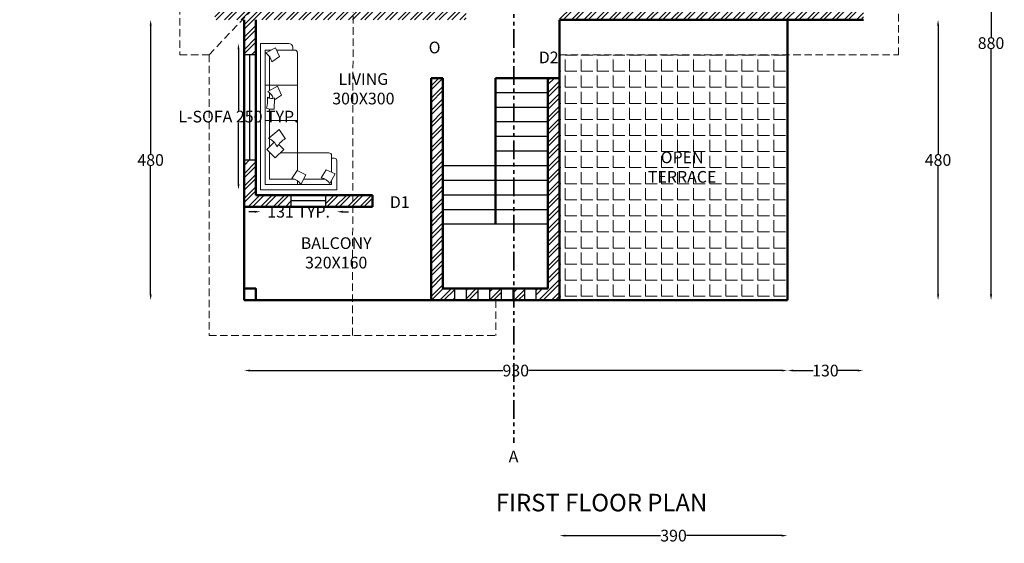
# Model space of a CAD drawing. Units: centimetres. Extents: x 10444 to 13814, y 8288 to 11191.
# Tile 8 of 9: x 12129 to 13814, y 9505 to 10401. Entities that reach past the tile are written whole.
import ezdxf

# ---------------------------------------------------------------- set-up
doc = ezdxf.new("R2010")
doc.units = ezdxf.units.CM
doc.header["$MEASUREMENT"] = 0
doc.linetypes.add('DASHED', pattern=[19.05, 12.7, -6.35])
doc.linetypes.add('PHANTOM', pattern=[63.5, 31.75, -6.35, 6.35, -6.35, 6.35, -6.35])
for name, color, linetype, lineweight in [('A-ANNO-DIMS', 2, 'Continuous', 18), ('A-ANNO-SYMB', 7, 'Continuous', 25), ('A-ANNO-SYMB-SECT', 1, 'PHANTOM', 35), ('A-ANNO-TEXT', 7, 'Continuous', 25), ('A-AREA-IDEN', 3, 'Continuous', 25), ('A-FLOR-PATT', 252, 'Continuous', 13), ('A-FLOR-STRS', 3, 'Continuous', 25), ('A-FURN', 8, 'Continuous', 18), ('A-GLAZ', 4, 'Continuous', 25), ('A-ROOF-OVHD', 6, 'DASHED', 18), ('A-WALL', 7, 'Continuous', 50), ('A-WALL-PATT', 8, 'Continuous', 13)]:
    doc.layers.add(name, color=color, linetype=linetype, lineweight=lineweight)
doc.styles.get("Standard").update_dxf_attribs({"font": 'arial.ttf'})
doc.dimstyles.get("Standard").update_dxf_attribs({"dimtxt": 20, "dimasz": 10, "dimexe": 0.18, "dimexo": 0.0625, "dimgap": 0.09, "dimtad": 0, "dimtih": 1, "dimtoh": 1, "dimdec": 0, "dimzin": 0, "dimdsep": 46, "dimtxsty": 'Standard', "dimcen": 0.09, "dimse1": 1, "dimse2": 1, "dimadec": 0, "dimazin": 0, "dimtfac": 1, "dimtdec": 0, "dimtofl": 0, "dimtmove": 0, "dimatfit": 3, "dimfxl": 1, "dimtolj": 1, "dimtzin": 0, "dimarcsym": 0})

# ---------------------------------------------------------------- blocks, each defined once
blk = doc.blocks.new('s')
at = {"color": 0, "linetype": 'ByBlock'}
for p, q in [((3164.2, 840.3), (3164.2, 844.8)), ((3171, 851.6), (3219.5, 851.6)), ((3186.7, 829.1), (3193.7, 844.2)), ((3193.7, 844.2), (3210.3, 835.3)), ((3219.5, 851.6), (3219.5, 601.2)), ((3156.3, 633.9), (3156.3, 835.8)), ((3160.9, 840.3), (3164.2, 840.3)), ((3191.9, 840.3), (3164.2, 840.3)), ((3200.2, 820.2), (3186.7, 829.1)), ((3211.6, 840.3), (3200.9, 840.3)), ((3203.7, 840.3), (3203.7, 838.8)), ((3203.7, 828.9), (3203.7, 771.1)), ((3211.6, 610.2), (3211.6, 840.3)), ((3156.3, 780.2), (3211.6, 780.2)), ((3183.2, 763.2), (3190.2, 778.3)), ((3190.2, 778.3), (3206.8, 769.4)), ((3195.3, 755.2), (3183.2, 763.2)), ((3203.7, 767.1), (3203.7, 757.8)), ((3196, 739.2), (3195.2, 758.2)), ((3203.7, 739.5), (3203.7, 674.9)), ((3156.3, 720), (3211.6, 720)), ((3187.4, 704.3), (3176.9, 688.9)), ((3205.6, 688.9), (3187.4, 704.3)), ((3188.2, 678.8), (3179.6, 670.3)), ((3208.3, 670.3), (3195.9, 682.7)), ((3097.7, 631.1), (3097.7, 659.8)), ((3102.2, 664.4), (3156.3, 664.4)), ((3156.3, 633.9), (3156.3, 664.4)), ((3156.3, 664.4), (3185.5, 664.4)), ((3179.6, 670.3), (3194, 655.9)), ((3194, 655.9), (3208.3, 670.3)), ((3203.7, 665.7), (3203.7, 619.2)), ((3088.7, 601.2), (3088.7, 650.8)), ((3093.2, 655.3), (3097.7, 655.3)), ((3106.7, 635.3), (3091.6, 628.3)), ((3091.6, 628.3), (3100.5, 611.7)), ((3115.6, 621.8), (3106.7, 635.3)), ((3156.6, 634), (3141.5, 627)), ((3141.5, 627), (3150.4, 610.4)), ((3165.5, 620.5), (3156.6, 634)), ((3097.7, 610.2), (3097.7, 616.9)), ((3156.3, 610.2), (3097.7, 610.2)), ((3145.7, 619.2), (3108.5, 619.2)), ((3156.3, 610.2), (3156.3, 616.7)), ((3156.3, 610.2), (3156.3, 616.7)), ((3211.6, 610.2), (3156.3, 610.2)), ((3203.7, 619.2), (3161.1, 619.2)), ((3156.3, 601.2), (3088.7, 601.2)), ((3219.5, 601.2), (3156.3, 601.2))]:
    blk.add_line(p, q, dxfattribs=at)
for centre, radius, start, end in [((3171, 844.8), 6.77, 90, 180), ((3160.9, 835.8), 4.51, 90, 180), ((3222.3, 816.3), 22.4, 122.3301, 170.157), ((3200.1, 772.4), 15, 250.8325, 299.9235), ((3218.8, 750.5), 22.4, 122.3301, 161.5057), ((3265.7, 754.9), 58.3, 175.599, 194.0402), ((3198.7, 772.8), 33.7, 265.4155, 288.0697), ((3153.1, 650.8), 44.9, 31.9301, 58.0699), ((3212.5, 667.6), 22.4, 108.0785, 161.9215), ((3102.2, 659.8), 4.51, 90, 180), ((3093.2, 650.8), 4.51, 90, 180), ((3119.4, 599.7), 22.4, 99.843, 147.6699), ((3169.3, 598.4), 22.4, 99.843, 147.6699)]:
    blk.add_arc(centre, radius, start, end, dxfattribs=at)
blk = doc.blocks.new('*D17')
at = {"layer": 'A-ANNO-DIMS', "color": 0, "lineweight": -2, "transparency": 16777216}
for p, q in [((12353.1, 10390.6), (12353.1, 10170.9)), ((12353.1, 9930.6), (12353.1, 10150.3))]:
    blk.add_line(p, q, dxfattribs=at)
at = {"layer": 'A-ANNO-DIMS', "color": 0, "transparency": 16777216}
for points in [[(12351.5, 10390.6), (12354.8, 10390.6), (12353.1, 10400.6)], [(12351.5, 9930.6), (12354.8, 9930.6), (12353.1, 9920.6)]]:
    blk.add_solid(points, dxfattribs=at)
at = {"layer": 'Defpoints', "color": 0, "transparency": 16777216}
for p in [(12353.1, 10400.6), (12513.1, 10400.6), (12513.1, 9920.6)]:
    blk.add_point(p, dxfattribs=at)
at = {"layer": 'A-ANNO-DIMS', "color": 0, "transparency": 16777216, "insert": (12353.1, 10160.6), "char_height": 20, "attachment_point": 5}
blk.add_mtext('\\A1;480', dxfattribs=at)
blk = doc.blocks.new('*D19')
at = {"layer": 'A-ANNO-DIMS', "color": 0, "lineweight": -2, "transparency": 16777216}
for p, q in [((13700.9, 10390.6), (13700.9, 10170.9)), ((13700.9, 9930.6), (13700.9, 10150.3))]:
    blk.add_line(p, q, dxfattribs=at)
at = {"layer": 'A-ANNO-DIMS', "color": 0, "transparency": 16777216}
for points in [[(13699.3, 10390.6), (13702.6, 10390.6), (13700.9, 10400.6)], [(13699.3, 9930.6), (13702.6, 9930.6), (13700.9, 9920.6)]]:
    blk.add_solid(points, dxfattribs=at)
at = {"layer": 'Defpoints', "color": 0, "transparency": 16777216}
for p in [(13443.1, 10400.6), (13443.1, 9920.6), (13700.9, 9920.6)]:
    blk.add_point(p, dxfattribs=at)
at = {"layer": 'A-ANNO-DIMS', "color": 0, "transparency": 16777216, "insert": (13700.9, 10160.6), "char_height": 20, "attachment_point": 5}
blk.add_mtext('\\A1;480', dxfattribs=at)
blk = doc.blocks.new('*D20')
at = {"layer": 'A-ANNO-DIMS', "color": 0, "lineweight": -2, "transparency": 16777216}
for p, q in [((12523.1, 9800.4), (12956, 9800.4)), ((13433.1, 9800.4), (13000.3, 9800.4))]:
    blk.add_line(p, q, dxfattribs=at)
at = {"layer": 'A-ANNO-DIMS', "color": 0, "transparency": 16777216}
for points in [[(12523.1, 9802.1), (12523.1, 9798.8), (12513.1, 9800.4)], [(13433.1, 9802.1), (13433.1, 9798.8), (13443.1, 9800.4)]]:
    blk.add_solid(points, dxfattribs=at)
at = {"layer": 'Defpoints', "color": 0, "transparency": 16777216}
for p in [(12513.1, 9920.6), (13443.1, 9920.6), (13443.1, 9800.4)]:
    blk.add_point(p, dxfattribs=at)
at = {"layer": 'A-ANNO-DIMS', "color": 0, "transparency": 16777216, "insert": (12978.1, 9800.4), "char_height": 20, "attachment_point": 5}
blk.add_mtext('\\A1;930', dxfattribs=at)
blk = doc.blocks.new('*D21')
at = {"layer": 'A-ANNO-DIMS', "color": 0, "lineweight": -2, "transparency": 16777216}
for p, q in [((13453.1, 9800.4), (13486.9, 9800.4)), ((13563.1, 9800.4), (13529.3, 9800.4))]:
    blk.add_line(p, q, dxfattribs=at)
at = {"layer": 'A-ANNO-DIMS', "color": 0, "transparency": 16777216}
for points in [[(13453.1, 9802.1), (13453.1, 9798.8), (13443.1, 9800.4)], [(13563.1, 9802.1), (13563.1, 9798.8), (13573.1, 9800.4)]]:
    blk.add_solid(points, dxfattribs=at)
at = {"layer": 'Defpoints', "color": 0, "transparency": 16777216}
for p in [(13443.1, 10400.6), (13573.1, 10400.6), (13443.1, 9800.4)]:
    blk.add_point(p, dxfattribs=at)
at = {"layer": 'A-ANNO-DIMS', "color": 0, "transparency": 16777216, "insert": (13508.1, 9800.4), "char_height": 20, "attachment_point": 5}
blk.add_mtext('\\A1;130', dxfattribs=at)
blk = doc.blocks.new('f')
for p, q in [((11304.7, 9881.5), (11164.7, 9881.5)), ((11164.7, 9881.5), (11164.7, 9861.5)), ((11184.7, 9881.5), (11184.7, 9861.5)), ((11204.7, 9881.5), (11204.7, 9861.5)), ((11224.7, 9881.5), (11224.7, 9861.5)), ((11244.7, 9881.5), (11244.7, 9861.5)), ((11264.7, 9881.5), (11264.7, 9861.5)), ((11284.7, 9881.5), (11284.7, 9861.5)), ((11304.7, 9861.5), (11304.7, 9881.5)), ((11164.7, 9861.5), (11304.7, 9861.5))]:
    blk.add_line(p, q)
blk = doc.blocks.new('WIN-1800')
blk.add_line((0, 10), (180, 10))
blk.add_lwpolyline([(0, 0), (180, 0), (180, 20), (0, 20)], close=True)
blk = doc.blocks.new('WIN-600')
blk.add_line((60, 10), (0, 10))
blk.add_lwpolyline([(0, 0), (60, 0), (60, 20), (0, 20)], close=True)
blk = doc.blocks.new('*D43')
at = {"layer": 'A-ANNO-DIMS', "color": 0, "lineweight": -2, "transparency": 16777216}
for p, q in [((12503.4, 10350.1), (12503.4, 10245.3)), ((12503.4, 10119.7), (12503.4, 10224.4))]:
    blk.add_line(p, q, dxfattribs=at)
at = {"layer": 'A-ANNO-DIMS', "color": 0, "transparency": 16777216}
for points in [[(12501.8, 10350.1), (12505.1, 10350.1), (12503.4, 10360.1)], [(12501.8, 10119.7), (12505.1, 10119.7), (12503.4, 10109.7)]]:
    blk.add_solid(points, dxfattribs=at)
at = {"layer": 'Defpoints', "color": 0, "transparency": 16777216}
for p in [(12503.4, 10360.1), (12541, 10360.1), (12541, 10109.7)]:
    blk.add_point(p, dxfattribs=at)
at = {"layer": 'A-ANNO-DIMS', "color": 0, "transparency": 16777216, "insert": (12503.4, 10234.9), "char_height": 20, "attachment_point": 5}
blk.add_mtext('\\A1;L-SOFA 250 TYP.', dxfattribs=at)
blk = doc.blocks.new('*D44')
at = {"layer": 'A-ANNO-DIMS', "color": 0, "lineweight": -2, "transparency": 16777216}
for p, q in [((12531, 10072.1), (12521, 10072.1)), ((12681.8, 10072.1), (12691.8, 10072.1))]:
    blk.add_line(p, q, dxfattribs=at)
at = {"layer": 'A-ANNO-DIMS', "color": 0, "transparency": 16777216}
for points in [[(12531, 10073.8), (12531, 10070.4), (12541, 10072.1)], [(12681.8, 10073.8), (12681.8, 10070.4), (12671.8, 10072.1)]]:
    blk.add_solid(points, dxfattribs=at)
at = {"layer": 'Defpoints', "color": 0, "transparency": 16777216}
for p in [(12541, 10109.7), (12671.8, 10109.7), (12541, 10072.1)]:
    blk.add_point(p, dxfattribs=at)
at = {"layer": 'A-ANNO-DIMS', "color": 0, "transparency": 16777216, "insert": (12606.4, 10072.1), "char_height": 20, "attachment_point": 5}
blk.add_mtext('\\A1;131 TYP.', dxfattribs=at)
blk = doc.blocks.new('*D66')
at = {"layer": 'A-ANNO-DIMS', "color": 0, "lineweight": -2, "transparency": 16777216}
for p, q in [((13791.6, 10790.6), (13791.6, 10370.9)), ((13791.6, 9930.6), (13791.6, 10350.3))]:
    blk.add_line(p, q, dxfattribs=at)
at = {"layer": 'A-ANNO-DIMS', "color": 0, "transparency": 16777216}
for points in [[(13789.9, 10790.6), (13793.3, 10790.6), (13791.6, 10800.6)], [(13789.9, 9930.6), (13793.3, 9930.6), (13791.6, 9920.6)]]:
    blk.add_solid(points, dxfattribs=at)
at = {"layer": 'Defpoints', "color": 0, "transparency": 16777216}
for p in [(13573.1, 10800.6), (13443.1, 9920.6), (13791.6, 9920.6)]:
    blk.add_point(p, dxfattribs=at)
at = {"layer": 'A-ANNO-DIMS', "color": 0, "transparency": 16777216, "insert": (13791.6, 10360.6), "char_height": 20, "attachment_point": 5}
blk.add_mtext('\\A1;880', dxfattribs=at)
blk = doc.blocks.new('*D83')
at = {"layer": 'A-ANNO-DIMS', "color": 0, "lineweight": -2, "transparency": 16777216}
for p, q in [((13063.1, 9518), (13226, 9518)), ((13433.1, 9518), (13270.2, 9518))]:
    blk.add_line(p, q, dxfattribs=at)
at = {"layer": 'A-ANNO-DIMS', "color": 0, "transparency": 16777216}
for points in [[(13063.1, 9519.7), (13063.1, 9516.3), (13053.1, 9518)], [(13433.1, 9519.7), (13433.1, 9516.3), (13443.1, 9518)]]:
    blk.add_solid(points, dxfattribs=at)
at = {"layer": 'Defpoints', "color": 0, "transparency": 16777216}
for p in [(13053.1, 9920.6), (13443.1, 9920.6), (13443.1, 9518)]:
    blk.add_point(p, dxfattribs=at)
at = {"layer": 'A-ANNO-DIMS', "color": 0, "transparency": 16777216, "insert": (13248.1, 9518), "char_height": 20, "attachment_point": 5}
blk.add_mtext('\\A1;390', dxfattribs=at)

msp = doc.modelspace()

# ---------------------------------------------------------------- hatches: boundary and pattern name
at = {"layer": 'A-FLOR-PATT'}
h = msp.add_hatch(dxfattribs=at)
h.set_pattern_fill('ANGLE', color=256, scale=100)
h.set_pattern_definition([(0, (0, 0), (0, 27.5), [20, -7.5]), (90, (0, 0), (-27.5, 2e-15), [20, -7.5])])
h.paths.add_polyline_path([(13443.1062, 10340.6336), (13053.1062, 10340.6336), (13053.1062, 10300.6336), (13053.1062, 9920.6336), (13443.1062, 9920.6336)])
h.paths.add_polyline_path([(13191.5444, 10110.203), (13335.0506, 10110.203), (13335.0506, 10185.0915), (13191.5444, 10185.0915)], flags=24)
at = {"layer": 'A-WALL-PATT'}
h = msp.add_hatch(dxfattribs=at)
h.set_pattern_fill('ANSI32', color=256, scale=40)
h.paths.add_polyline_path([(12933.1062, 10800.6336), (12768.1062, 10800.6336), (12768.1062, 10780.6336), (12933.1062, 10780.6336)])
h.paths.add_polyline_path([(12588.1062, 10800.6336), (12463.1062, 10800.6336), (12463.1062, 10780.6336), (12588.1062, 10780.6336)])
h.paths.add_polyline_path([(12483.1062, 10726.41), (12483.1062, 10780.6336), (12463.1062, 10780.6336), (12463.1062, 10690.6336), (12483.1062, 10690.6336)])
h.paths.add_polyline_path([(12483.1062, 10510.6336), (12463.1062, 10510.6336), (12463.1062, 10400.6336), (12510.094, 10400.6336), (12529.0899, 10420.6336), (12483.1062, 10420.6336)])
h.paths.add_polyline_path([(12699.6814, 10420.6336), (12529.0899, 10420.6336), (12510.094, 10400.6336), (12513.1062, 10400.6336), (12513.1062, 10340.6336), (12533.1062, 10340.6336), (12533.1062, 10400.6336), (12699.64, 10400.6336)])
h.paths.add_polyline_path([(12893.1062, 10420.6336), (12699.6814, 10420.6336), (12699.64, 10400.6336), (12893.1062, 10400.6336)])
h.paths.add_polyline_path([(13129.7438, 10800.6336), (12993.1062, 10800.6336), (12993.1062, 10780.6336), (13033.1062, 10780.6336), (13033.1062, 10600.6336), (13053.1062, 10600.6336), (13053.1062, 10780.6336), (13129.7438, 10780.6336)])
h.paths.add_polyline_path([(13433.1062, 10800.6336), (13309.7438, 10800.6336), (13309.7438, 10780.6336), (13345.5201, 10780.6336), (13353.1062, 10780.6336), (13353.1062, 10600.6336), (13373.1062, 10600.6336), (13373.1062, 10780.6336), (13433.1062, 10780.6336)])
h.paths.add_polyline_path([(13573.1062, 10800.6336), (13493.1062, 10800.6336), (13493.1062, 10780.6336), (13553.1062, 10780.6336), (13553.1062, 10600.6336), (13573.1062, 10600.6336)])
h.paths.add_polyline_path([(13573.1062, 10600.6336), (13553.1062, 10600.6336), (13553.1062, 10420.6336), (13053.1062, 10420.6336), (13053.1062, 10400.6336), (13573.1062, 10400.6336)])
h.paths.add_polyline_path([(13053.1062, 10300.6336), (13033.1062, 10300.6336), (13033.1062, 9940.6336), (13013.1062, 9940.6336), (13013.1062, 9920.6336), (13053.1062, 9920.6336)])
h.paths.add_polyline_path([(12993.1062, 9940.6336), (12975, 9940.6336), (12975, 9920.6336), (12993.1062, 9920.6336)])
h.paths.add_polyline_path([(12953.1062, 9940.6336), (12933.1062, 9940.6336), (12933.1062, 9920.6336), (12953.1062, 9920.6336)])
h.paths.add_polyline_path([(12913.1062, 9940.6336), (12893.1062, 9940.6336), (12893.1062, 9920.6336), (12913.1062, 9920.6336)])
h.paths.add_polyline_path([(12873.1062, 9940.6336), (12853.1062, 9940.6336), (12853.1062, 10300.6336), (12833.1062, 10300.6336), (12833.1062, 9920.6336), (12873.1062, 9920.6336)])
h.paths.add_polyline_path([(12733.1062, 10100.6336), (12699.0201, 10100.6336), (12698.9788, 10080.6336), (12733.1062, 10080.6336)])
h.paths.add_polyline_path([(12699.0201, 10100.6336), (12653.1062, 10100.6336), (12653.1062, 10080.6336), (12698.9788, 10080.6336)])
h.paths.add_polyline_path([(12593.1062, 10100.6336), (12533.1062, 10100.6336), (12533.1062, 10160.6336), (12513.1062, 10160.6336), (12513.1062, 10080.6336), (12593.1062, 10080.6336)])
h.paths.add_polyline_path([(13053.1062, 10600.6336), (13033.1062, 10600.6336), (13033.1062, 10576.2537, -0.004993085), (13033.1062, 10574.2995), (13033.1062, 10564.3331, -0.269473124), (13034.9053, 10565.2433), (13034.9053, 10561.5839), (13034.9053, 10557.6884, -0.269473124), (13033.1062, 10558.5987), (13033.1062, 10530.6336), (12975, 10530.6336), (12975, 10510.6336), (13053.1062, 10510.6336)])
h.paths.add_polyline_path([(12975, 10530.6336), (12893.1062, 10530.6336), (12893.1062, 10600.6336), (12873.1062, 10600.6336), (12873.1062, 10510.6336), (12975, 10510.6336)])
h.paths.add_polyline_path([(12893.1062, 10700.6336), (12873.1062, 10700.6336), (12873.1062, 10600.6336), (12893.1062, 10600.6336)])
h.paths.add_polyline_path([(13373.1062, 10600.6336), (13353.1062, 10600.6336), (13353.1062, 10507.9506), (13373.1062, 10507.9506)], flags=17)
h.paths.add_polyline_path([(13553.1062, 10620.6336), (13453.1062, 10620.6336), (13453.1062, 10600.6336), (13553.1062, 10600.6336)])
h.paths.add_polyline_path([(11114.7881, 10700.6336), (11094.7881, 10700.6336), (11094.7881, 10510.6336), (11196.6819, 10510.6336), (11196.6819, 10530.6336), (11114.7881, 10530.6336)])

# ---------------------------------------------------------------- linework, layer by layer
at = {"layer": 'A-ANNO-SYMB-SECT'}
msp.add_line((12975, 11019.5), (12975, 9676.5), dxfattribs=at)
at = {"layer": 'A-FLOR-STRS'}
for p, q in [((13033.1062, 10275.6336), (12943.1062, 10275.6336)), ((13033.1062, 10250.6336), (12943.1062, 10250.6336)), ((13033.1062, 10225.6336), (12943.1062, 10225.6336)), ((13033.1062, 10200.6336), (12943.1062, 10200.6336)), ((13033.1062, 10175.6336), (12943.1062, 10175.6336)), ((13033.1062, 10150.6336), (12853.1062, 10150.6336)), ((13033.1062, 10125.6336), (12853.1062, 10125.6336)), ((13033.1062, 10100.6336), (12853.1062, 10100.6336)), ((13033.1062, 10075.6336), (12853.1062, 10075.6336)), ((13033.1062, 10050.6336), (12853.1062, 10050.6336))]:
    msp.add_line(p, q, dxfattribs=at)
at = {"layer": 'A-ROOF-OVHD'}
for p, q in [((12403.1062, 10860.6336), (12403.1062, 10340.6336)), ((13633.1062, 10340.6336), (13633.1062, 10860.6336)), ((12453.1062, 10340.6336), (12700.0533, 10600.6336)), ((12698.5242, 9860.6336), (12700.0533, 10600.6336)), ((12403.1062, 10340.6336), (12453.1062, 10340.6336)), ((12453.1062, 10340.6336), (12453.1062, 9860.6336)), ((13053.1062, 10340.6336), (13633.1062, 10340.6336)), ((12943.9422, 9920.6336), (12943.9422, 9860.6336)), ((12453.1062, 9860.6336), (12943.9422, 9860.6336))]:
    msp.add_line(p, q, dxfattribs=at)
at = {"layer": 'A-WALL'}
for p, q in [((12513.1062, 10400.6336), (12513.1062, 9920.6336)), ((12533.1062, 10400.6336), (12533.1062, 10100.6336)), ((13053.1062, 10400.6336), (13573.1062, 10400.6336)), ((13053.1062, 10400.6336), (13053.1062, 10300.6336)), ((13443.1062, 9920.6336), (13443.1062, 10400.6336)), ((12833.1062, 10300.6336), (12833.1062, 9920.6336)), ((12853.1062, 10300.6336), (12833.1062, 10300.6336)), ((12853.1062, 10300.6336), (12853.1062, 9940.6336)), ((13033.1062, 10300.6336), (12943.1062, 10300.6336)), ((12943.1062, 10300.6336), (12943.1062, 10050.6336)), ((13033.1062, 10300.6336), (13033.1062, 9940.6336)), ((13053.1062, 10300.6336), (13033.1062, 10300.6336)), ((13053.1062, 10300.6336), (13053.1062, 9920.6336)), ((12533.1062, 10100.6336), (12733.1062, 10100.6336)), ((12733.1062, 10100.6336), (12733.1062, 10080.6336)), ((12513.1062, 10080.6336), (12733.1062, 10080.6336)), ((13033.1062, 9940.6336), (12853.1062, 9940.6336)), ((12513.1062, 9920.6336), (13443.1062, 9920.6336))]:
    msp.add_line(p, q, dxfattribs=at)
msp.add_lwpolyline([(12513.1062, 9920.6336), (12533.1062, 9920.6336), (12533.1062, 9940.6336), (12513.1062, 9940.6336)], close=True, dxfattribs=at)

# ---------------------------------------------------------------- block references
at = {"layer": 'A-FURN', "xscale": -1}
msp.add_blockref('s', (15760.519, 9508.4652), dxfattribs=at)
at = {"layer": 'A-GLAZ', "rotation": 90}
msp.add_blockref('WIN-1800', (12533.1058, 10160.6335), dxfattribs=at)
at = {"layer": 'A-GLAZ'}
for name, p in [('WIN-600', (12593.1061, 10080.634)), ('f', (1708.4374, 59.1341))]:
    msp.add_blockref(name, p, dxfattribs=at)

# ---------------------------------------------------------------- texts
at = {"layer": 'A-ANNO-SYMB', "insert": (12966, 9663.5), "char_height": 20, "attachment_point": 1}
msp.add_mtext_dynamic_manual_height_columns('A', width=668.5, gutter_width=1, heights=[0], dxfattribs=at)
at = {"layer": 'A-ANNO-TEXT', "attachment_point": 1}
for s, width, insert, char_height in [('O', 668.5, (12828.9845, 10363.1095), 20), ('D2', 668.5, (13017.5, 10346.0819), 20), ('D1', 668.5, (12762.537, 10098.5819), 20), ('\\pxqc;FIRST FLOOR PLAN', 406.387623, (12921.6808, 9589.5), 30)]:
    msp.add_mtext_dynamic_manual_height_columns(s, width=width, gutter_width=1, heights=[0], dxfattribs=dict(at, insert=insert, char_height=char_height))
at = {"layer": 'A-AREA-IDEN', "char_height": 20, "attachment_point": 1}
for s, insert in [('\\pxqc;LIVING\\P300X300', (12642.9224, 10309.0931)), ('\\pxqc;OPEN TERRACE', (13188.5537, 10175.1529)), ('\\pxqc;BALCONY\\P320X160', (12596.3779, 10028.404))]:
    msp.add_mtext_dynamic_manual_height_columns(s, width=148.64167, gutter_width=1, heights=[0], dxfattribs=dict(at, insert=insert))

# ---------------------------------------------------------------- dimensions: what is measured, and where the dimension line sits
at = {"layer": 'A-ANNO-DIMS'}
dim = msp.add_linear_dim(base=(13791.6062, 9920.6336), p1=(13573.1062, 10800.6336), p2=(13443.1062, 9920.6336), angle=90, dimstyle='Standard', override={"dimdec": 0, "dimlfac": 1, "dimrnd": 0, "dimzin": 0, "dimdsep": 46, "dimlunit": 2}, dxfattribs=at)
dim.commit()
dim.dimension.update_dxf_attribs({"geometry": '*D66', "text_midpoint": (13791.6062, 10360.6336)})
for p1, p2, distance, picture, middle in [((12513.1062, 9920.6336), (12513.1062, 10400.6336), 159.9671, '*D17', (12353.1391, 10160.6336)), ((13443.1062, 10400.6336), (13443.1062, 9920.6336), 257.8354, '*D19', (13700.9416, 10160.6336)), ((13573.1062, 10400.6336), (13443.1062, 10400.6336), 600.2041, '*D21', (13508.1062, 9800.4295)), ((12513.1062, 9920.6336), (13443.1062, 9920.6336), -120.2041, '*D20', (12978.1062, 9800.4295))]:
    dim = msp.add_aligned_dim(p1=p1, p2=p2, distance=distance, dimstyle='Standard', override={"dimclrd": 0, "dimclre": 0, "dimclrt": 0}, dxfattribs=at)
    dim.commit()
    dim.dimension.update_dxf_attribs({"geometry": picture, "text_midpoint": middle})
for base, p1, p2, angle, text, picture, middle in [((12503.4399, 10360.0729), (12541.0022, 10109.6576), (12541.0022, 10360.0729), 90, 'L-SOFA <> TYP.', '*D43', (12503.4399, 10234.8653)), ((12541.0022, 10072.0953), (12671.8498, 10109.6576), (12541.0022, 10109.6576), 180, '<> TYP.', '*D44', (12606.426, 10072.0953))]:
    dim = msp.add_linear_dim(base=base, p1=p1, p2=p2, angle=angle, text=text, dimstyle='Standard', override={"dimdec": 0, "dimrnd": 0, "dimzin": 0, "dimlunit": 2}, dxfattribs=at)
    dim.commit()
    dim.dimension.update_dxf_attribs({"geometry": picture, "text_midpoint": middle})
dim = msp.add_linear_dim(base=(13443.1062, 9518), p1=(13053.1062, 9920.6336), p2=(13443.1062, 9920.6336), dimstyle='Standard', override={"dimdec": 0, "dimlfac": 1, "dimrnd": 0, "dimzin": 0, "dimdsep": 46, "dimlunit": 2}, dxfattribs=at)
dim.commit()
dim.dimension.update_dxf_attribs({"geometry": '*D83', "text_midpoint": (13248.1062, 9518)})

doc.saveas('drawing.dxf')
